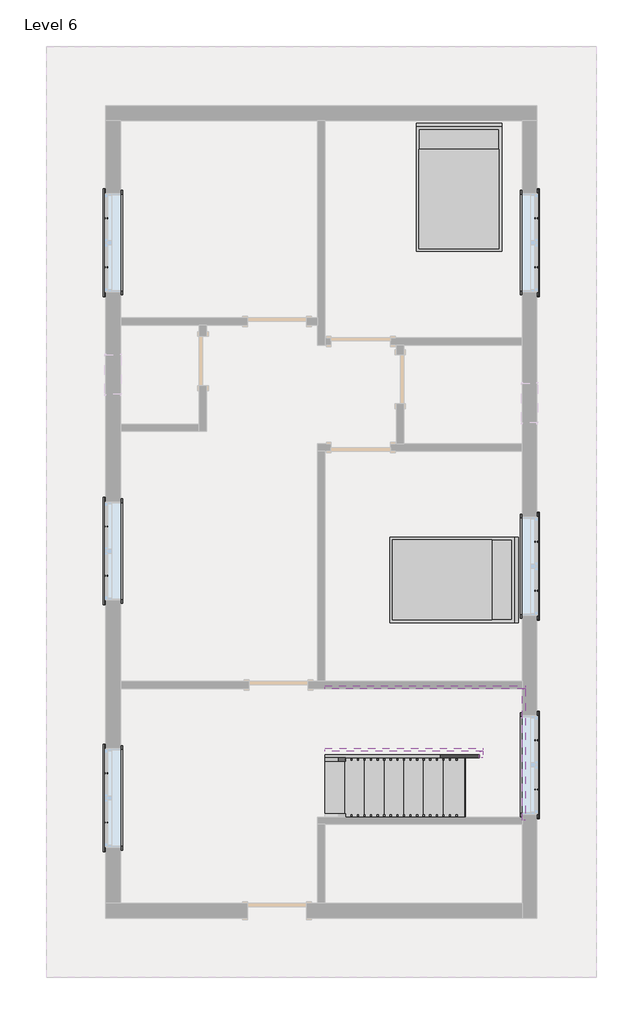
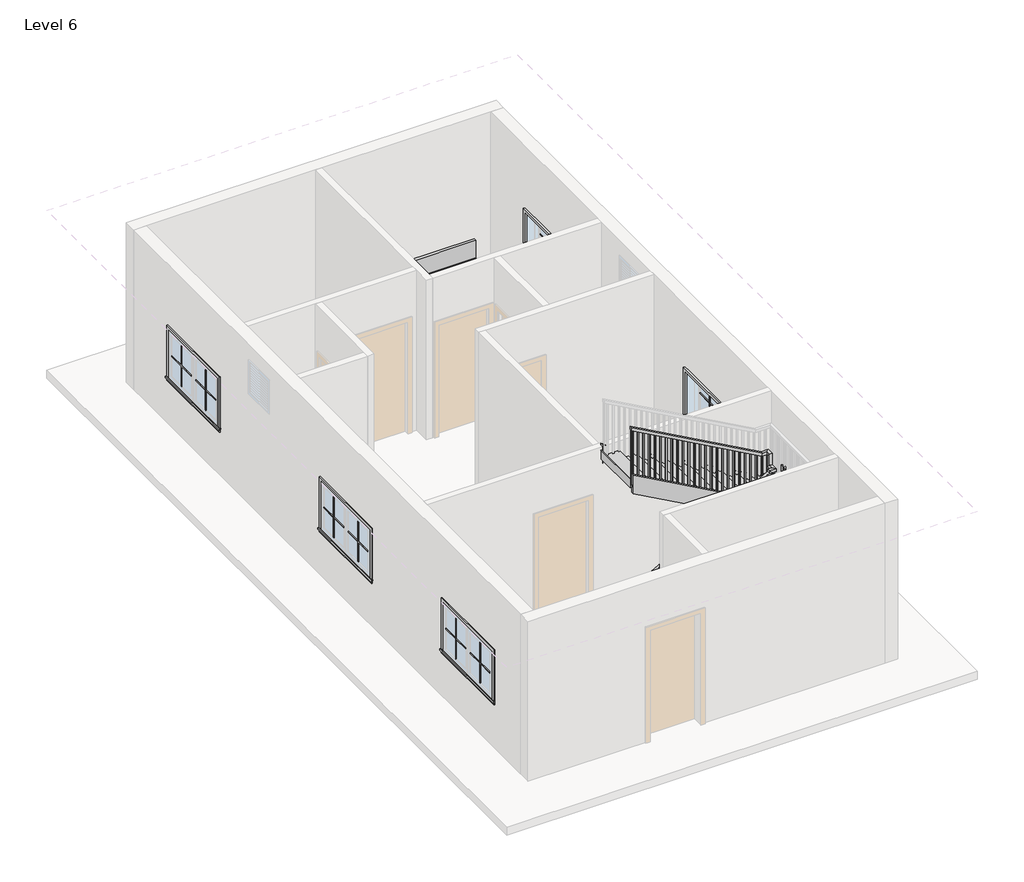
# One storey, part 3 of 3: 24 proxies, 6 members, 2 furniture elements, 1 railing, 1 stair flight.
"""IFC4 building model written with IfcOpenShell, lengths in millimetres."""

from ifc_helpers import new_model, si_unit, frame, origin, place, context, project, spatial, polyline, outline, extrude, faceted_brep, transform, mapped, element, save
from components import muntin_pattern_2x2_muntin_pattern_2x2_9352d081, muntin_pattern_2x2_muntin_pattern_2x2_5c2cbe28, trim_window_exterior_flat_with_sill_979bde60, trim_window_interior_flat_picture_frame_7883d11b, bed_17739_bed_17739_15c61121, stair_flight_3ef849b5

model = new_model("IFC4")

# Units and contexts
model_context = context("Model", 3, world=origin())
ifc_project = project(units=[si_unit("LENGTHUNIT", "METRE", prefix="MILLI")], contexts=[model_context])

# Site, building, storey
site = spatial("IfcSite", under=ifc_project)
building = spatial("IfcBuilding", under=site)
storey = spatial("IfcBuildingStorey", under=building, Name="Level 6", Elevation=15849.6)

# Proxies
placement = place(None, origin())
muntin_pattern_2x2_muntin_pattern_2x2_shape = muntin_pattern_2x2_muntin_pattern_2x2_9352d081(model_context)
element("IfcBuildingElementProxy", 1, Name="Muntin Pattern_2x2 : Muntin Pattern_2x2", ObjectType="Muntin Pattern_2x2 : Muntin Pattern_2x2", at=placement, inside=storey, context=model_context, shape_type="MappedRepresentation", body=[
    mapped(muntin_pattern_2x2_muntin_pattern_2x2_shape, transform((-4579.34688, 3675.02881, 16833.85), x_axis=(0.0, 1.0, 0.0), y_axis=(-1.0, 0.0, 0.0), z_axis=(0.0, 0.0, 1.0))),
])
element("IfcBuildingElementProxy", 2, Name="Muntin Pattern_2x2 : Muntin Pattern_2x2", ObjectType="Muntin Pattern_2x2 : Muntin Pattern_2x2", at=placement, inside=storey, context=model_context, shape_type="MappedRepresentation", body=[
    mapped(muntin_pattern_2x2_muntin_pattern_2x2_shape, transform((-4579.34688, -1087.47119, 16833.85), x_axis=(0.0, 1.0, 0.0), y_axis=(-1.0, 0.0, 0.0), z_axis=(0.0, 0.0, 1.0))),
])
element("IfcBuildingElementProxy", 3, Name="Muntin Pattern_2x2 : Muntin Pattern_2x2", ObjectType="Muntin Pattern_2x2 : Muntin Pattern_2x2", at=placement, inside=storey, context=model_context, shape_type="MappedRepresentation", body=[
    mapped(muntin_pattern_2x2_muntin_pattern_2x2_shape, transform((-4579.34688, -4900.64619, 16833.85), x_axis=(0.0, 1.0, 0.0), y_axis=(-1.0, 0.0, 0.0), z_axis=(0.0, 0.0, 1.0))),
])
element("IfcBuildingElementProxy", 4, Name="Muntin Pattern_2x2 : Muntin Pattern_2x2", ObjectType="Muntin Pattern_2x2 : Muntin Pattern_2x2", at=placement, inside=storey, context=model_context, shape_type="MappedRepresentation", body=[
    mapped(muntin_pattern_2x2_muntin_pattern_2x2_shape, transform((2069.10312, -3630.64619, 16833.85), x_axis=(0.0, -1.0, 0.0), y_axis=(1.0, 0.0, 0.0), z_axis=(0.0, 0.0, 1.0))),
])
element("IfcBuildingElementProxy", 5, Name="Muntin Pattern_2x2 : Muntin Pattern_2x2", ObjectType="Muntin Pattern_2x2 : Muntin Pattern_2x2", at=placement, inside=storey, context=model_context, shape_type="MappedRepresentation", body=[
    mapped(muntin_pattern_2x2_muntin_pattern_2x2_shape, transform((2069.10312, 4433.85381, 16833.85), x_axis=(0.0, -1.0, 0.0), y_axis=(1.0, 0.0, 0.0), z_axis=(0.0, 0.0, 1.0))),
])
element("IfcBuildingElementProxy", 6, Name="Muntin Pattern_2x2 : Muntin Pattern_2x2", ObjectType="Muntin Pattern_2x2 : Muntin Pattern_2x2", at=placement, inside=storey, context=model_context, shape_type="MappedRepresentation", body=[
    mapped(muntin_pattern_2x2_muntin_pattern_2x2_shape, transform((2069.10312, -563.59619, 16833.85), x_axis=(0.0, -1.0, 0.0), y_axis=(1.0, 0.0, 0.0), z_axis=(0.0, 0.0, 1.0))),
])
muntin_pattern_2x2_muntin_pattern_2x2_2_shape = muntin_pattern_2x2_muntin_pattern_2x2_5c2cbe28(model_context)
element("IfcBuildingElementProxy", 7, Name="Muntin Pattern_2x2 : Muntin Pattern_2x2", ObjectType="Muntin Pattern_2x2 : Muntin Pattern_2x2", at=placement, inside=storey, context=model_context, shape_type="MappedRepresentation", body=[
    mapped(muntin_pattern_2x2_muntin_pattern_2x2_2_shape, transform((-4579.34688, 4433.85381, 16833.85), x_axis=(0.0, -1.0, 0.0), y_axis=(1.0, 0.0, 0.0), z_axis=(0.0, 0.0, 1.0))),
])
element("IfcBuildingElementProxy", 8, Name="Muntin Pattern_2x2 : Muntin Pattern_2x2", ObjectType="Muntin Pattern_2x2 : Muntin Pattern_2x2", at=placement, inside=storey, context=model_context, shape_type="MappedRepresentation", body=[
    mapped(muntin_pattern_2x2_muntin_pattern_2x2_2_shape, transform((-4579.34688, -328.64619, 16833.85), x_axis=(0.0, -1.0, 0.0), y_axis=(1.0, 0.0, 0.0), z_axis=(0.0, 0.0, 1.0))),
])
element("IfcBuildingElementProxy", 9, Name="Muntin Pattern_2x2 : Muntin Pattern_2x2", ObjectType="Muntin Pattern_2x2 : Muntin Pattern_2x2", at=placement, inside=storey, context=model_context, shape_type="MappedRepresentation", body=[
    mapped(muntin_pattern_2x2_muntin_pattern_2x2_2_shape, transform((-4579.34688, -4141.82119, 16833.85), x_axis=(0.0, -1.0, 0.0), y_axis=(1.0, 0.0, 0.0), z_axis=(0.0, 0.0, 1.0))),
])
element("IfcBuildingElementProxy", 10, Name="Muntin Pattern_2x2 : Muntin Pattern_2x2", ObjectType="Muntin Pattern_2x2 : Muntin Pattern_2x2", at=placement, inside=storey, context=model_context, shape_type="MappedRepresentation", body=[
    mapped(muntin_pattern_2x2_muntin_pattern_2x2_2_shape, transform((2069.10312, -4389.47119, 16833.85), x_axis=(0.0, 1.0, 0.0), y_axis=(-1.0, 0.0, 0.0), z_axis=(0.0, 0.0, 1.0))),
])
element("IfcBuildingElementProxy", 11, Name="Muntin Pattern_2x2 : Muntin Pattern_2x2", ObjectType="Muntin Pattern_2x2 : Muntin Pattern_2x2", at=placement, inside=storey, context=model_context, shape_type="MappedRepresentation", body=[
    mapped(muntin_pattern_2x2_muntin_pattern_2x2_2_shape, transform((2069.10312, 3675.02881, 16833.85), x_axis=(0.0, 1.0, 0.0), y_axis=(-1.0, 0.0, 0.0), z_axis=(0.0, 0.0, 1.0))),
])
element("IfcBuildingElementProxy", 12, Name="Muntin Pattern_2x2 : Muntin Pattern_2x2", ObjectType="Muntin Pattern_2x2 : Muntin Pattern_2x2", at=placement, inside=storey, context=model_context, shape_type="MappedRepresentation", body=[
    mapped(muntin_pattern_2x2_muntin_pattern_2x2_2_shape, transform((2069.10312, -1322.42119, 16833.85), x_axis=(0.0, 1.0, 0.0), y_axis=(-1.0, 0.0, 0.0), z_axis=(0.0, 0.0, 1.0))),
])
trim_window_exterior_flat_with_sill_shape = trim_window_exterior_flat_with_sill_979bde60(model_context)
element("IfcBuildingElementProxy", 13, Name="Trim-Window-Exterior-Flat : with Sill", ObjectType="Trim-Window-Exterior-Flat : with Sill", at=placement, inside=storey, context=model_context, shape_type="MappedRepresentation", body=[
    mapped(trim_window_exterior_flat_with_sill_shape, transform((-4588.87188, 4054.44131, 17678.4), x_axis=(0.0, -1.0, 0.0), y_axis=(0.0, 0.0, 1.0), z_axis=(-1.0, 0.0, 0.0))),
])
element("IfcBuildingElementProxy", 14, Name="Trim-Window-Exterior-Flat : with Sill", ObjectType="Trim-Window-Exterior-Flat : with Sill", at=placement, inside=storey, context=model_context, shape_type="MappedRepresentation", body=[
    mapped(trim_window_exterior_flat_with_sill_shape, transform((-4588.87188, -708.05869, 17678.4), x_axis=(0.0, -1.0, 0.0), y_axis=(0.0, 0.0, 1.0), z_axis=(-1.0, 0.0, 0.0))),
])
element("IfcBuildingElementProxy", 15, Name="Trim-Window-Exterior-Flat : with Sill", ObjectType="Trim-Window-Exterior-Flat : with Sill", at=placement, inside=storey, context=model_context, shape_type="MappedRepresentation", body=[
    mapped(trim_window_exterior_flat_with_sill_shape, transform((-4588.87188, -4521.23369, 17678.4), x_axis=(0.0, -1.0, 0.0), y_axis=(0.0, 0.0, 1.0), z_axis=(-1.0, 0.0, 0.0))),
])
element("IfcBuildingElementProxy", 16, Name="Trim-Window-Exterior-Flat : with Sill", ObjectType="Trim-Window-Exterior-Flat : with Sill", at=placement, inside=storey, context=model_context, shape_type="MappedRepresentation", body=[
    mapped(trim_window_exterior_flat_with_sill_shape, transform((2078.62812, -4010.05869, 17678.4), x_axis=(0.0, 1.0, 0.0), y_axis=(0.0, 0.0, 1.0), z_axis=(1.0, 0.0, 0.0))),
])
element("IfcBuildingElementProxy", 17, Name="Trim-Window-Exterior-Flat : with Sill", ObjectType="Trim-Window-Exterior-Flat : with Sill", at=placement, inside=storey, context=model_context, shape_type="MappedRepresentation", body=[
    mapped(trim_window_exterior_flat_with_sill_shape, transform((2078.62812, 4054.44131, 17678.4), x_axis=(0.0, 1.0, 0.0), y_axis=(0.0, 0.0, 1.0), z_axis=(1.0, 0.0, 0.0))),
])
element("IfcBuildingElementProxy", 18, Name="Trim-Window-Exterior-Flat : with Sill", ObjectType="Trim-Window-Exterior-Flat : with Sill", at=placement, inside=storey, context=model_context, shape_type="MappedRepresentation", body=[
    mapped(trim_window_exterior_flat_with_sill_shape, transform((2078.62812, -943.00869, 17678.4), x_axis=(0.0, 1.0, 0.0), y_axis=(0.0, 0.0, 1.0), z_axis=(1.0, 0.0, 0.0))),
])
trim_window_interior_flat_picture_frame_shape = trim_window_interior_flat_picture_frame_7883d11b(model_context)
element("IfcBuildingElementProxy", 19, Name="Trim-Window-Interior-Flat : Picture Frame", ObjectType="Trim-Window-Interior-Flat : Picture Frame", at=placement, inside=storey, context=model_context, shape_type="MappedRepresentation", body=[
    mapped(trim_window_interior_flat_picture_frame_shape, transform((-4360.27188, 4054.44131, 17678.4), x_axis=(0.0, 1.0, 0.0), y_axis=(0.0, 0.0, 1.0), z_axis=(1.0, 0.0, 0.0))),
])
element("IfcBuildingElementProxy", 20, Name="Trim-Window-Interior-Flat : Picture Frame", ObjectType="Trim-Window-Interior-Flat : Picture Frame", at=placement, inside=storey, context=model_context, shape_type="MappedRepresentation", body=[
    mapped(trim_window_interior_flat_picture_frame_shape, transform((-4360.27188, -708.05869, 17678.4), x_axis=(0.0, 1.0, 0.0), y_axis=(0.0, 0.0, 1.0), z_axis=(1.0, 0.0, 0.0))),
])
element("IfcBuildingElementProxy", 21, Name="Trim-Window-Interior-Flat : Picture Frame", ObjectType="Trim-Window-Interior-Flat : Picture Frame", at=placement, inside=storey, context=model_context, shape_type="MappedRepresentation", body=[
    mapped(trim_window_interior_flat_picture_frame_shape, transform((-4360.27188, -4521.23369, 17678.4), x_axis=(0.0, 1.0, 0.0), y_axis=(0.0, 0.0, 1.0), z_axis=(1.0, 0.0, 0.0))),
])
element("IfcBuildingElementProxy", 22, Name="Trim-Window-Interior-Flat : Picture Frame", ObjectType="Trim-Window-Interior-Flat : Picture Frame", at=placement, inside=storey, context=model_context, shape_type="MappedRepresentation", body=[
    mapped(trim_window_interior_flat_picture_frame_shape, transform((1850.02812, -4010.05869, 17678.4), x_axis=(0.0, -1.0, 0.0), y_axis=(0.0, 0.0, 1.0), z_axis=(-1.0, 0.0, 0.0))),
])
element("IfcBuildingElementProxy", 23, Name="Trim-Window-Interior-Flat : Picture Frame", ObjectType="Trim-Window-Interior-Flat : Picture Frame", at=placement, inside=storey, context=model_context, shape_type="MappedRepresentation", body=[
    mapped(trim_window_interior_flat_picture_frame_shape, transform((1850.02812, 4054.44131, 17678.4), x_axis=(0.0, -1.0, 0.0), y_axis=(0.0, 0.0, 1.0), z_axis=(-1.0, 0.0, 0.0))),
])
element("IfcBuildingElementProxy", 24, Name="Trim-Window-Interior-Flat : Picture Frame", ObjectType="Trim-Window-Interior-Flat : Picture Frame", at=placement, inside=storey, context=model_context, shape_type="MappedRepresentation", body=[
    mapped(trim_window_interior_flat_picture_frame_shape, transform((1850.02812, -943.00869, 17678.4), x_axis=(0.0, -1.0, 0.0), y_axis=(0.0, 0.0, 1.0), z_axis=(-1.0, 0.0, 0.0))),
])

# Furniture
bed_17739_bed_17739_shape = bed_17739_bed_17739_15c61121(model_context)
element("IfcFurniture", 25, ObjectType="Bed_17739 : Bed_17739", at=placement, inside=storey, context=model_context, shape_type="MappedRepresentation", body=[
    mapped(bed_17739_bed_17739_shape, transform((872.12812, 4886.29131, 15849.6), x_axis=(1.0, 0.0, 0.0), y_axis=(0.0, 1.0, 0.0), z_axis=(0.0, 0.0, 1.0))),
])
element("IfcFurniture", 26, ObjectType="Bed_17739 : Bed_17739", at=placement, inside=storey, context=model_context, shape_type="MappedRepresentation", body=[
    mapped(bed_17739_bed_17739_shape, transform((770.52812, -1152.55869, 15849.6), x_axis=(0.0, -1.0, 0.0), y_axis=(1.0, 0.0, 0.0), z_axis=(0.0, 0.0, 1.0))),
])

# Members
element("IfcMember", 27, ObjectType="Stringer - 2\" Width", at=placement, inside=storey, context=model_context, shape_type="SweptSolid", body=[
    extrude(outline(polyline([(16057.1983948, -1197.97188), (15849.6, -1197.97188), (15849.6, -944.0273772), (17034.9641651, 1189.62812), (17383.6428392, 1189.62812), (16057.1983948, -1197.97188)])), frame((0.0, -3902.10869, 0.0), z_axis=(0.0, 1.0, 0.0), x_axis=(0.0, 0.0, 1.0)), (0.0, 0.0, 1.0), 50.8),
])
element("IfcMember", 28, ObjectType="Stringer - 2\" Width", at=placement, inside=storey, context=model_context, shape_type="SweptSolid", body=[
    extrude(outline(polyline([(1240.42812, -3902.10869), (1189.62812, -3902.10869), (1189.62812, -3800.50869), (1240.42812, -3800.50869), (1240.42812, -3902.10869)])), frame((0.0, 0.0, 17145.0), z_axis=(0.0, 0.0, 1.0), x_axis=(1.0, 0.0, 0.0)), (0.0, 0.0, 1.0), 304.8),
])
element("IfcMember", 29, ObjectType="Stringer - 2\" Width", at=placement, inside=storey, context=model_context, shape_type="SweptSolid", body=[
    extrude(outline(polyline([(17232.5197207, 1240.42812), (17581.1983948, 1240.42812), (18935.8650614, -1197.97188), (18587.1863873, -1197.97188), (17232.5197207, 1240.42812)])), frame((0.0, -3800.50869, 0.0), z_axis=(0.0, 1.0, 0.0), x_axis=(0.0, 0.0, 1.0)), (0.0, 0.0, 1.0), 50.8),
])
element("IfcMember", 30, ObjectType="Stringer - 2\" Width", at=placement, inside=storey, context=model_context, shape_type="SweptSolid", body=[
    extrude(outline(polyline([(16057.1983948, -1197.97188), (15849.6, -1197.97188), (15849.6, -944.0273772), (17401.853054, 1850.02812), (17449.8, 1850.02812), (17449.8, 1308.7110094), (16057.1983948, -1197.97188)])), frame((0.0, -4867.30869, 0.0), z_axis=(0.0, 1.0, 0.0), x_axis=(0.0, 0.0, 1.0)), (0.0, 0.0, 1.0), 50.8),
])
element("IfcMember", 31, ObjectType="Stringer - 2\" Width", at=placement, inside=storey, context=model_context, shape_type="SweptSolid", body=[
    extrude(outline(polyline([(1900.82812, -4867.30869), (1850.02812, -4867.30869), (1850.02812, -2835.30869), (1900.82812, -2835.30869), (1900.82812, -4867.30869)])), frame((0.0, 0.0, 17145.0), z_axis=(0.0, 0.0, 1.0), x_axis=(1.0, 0.0, 0.0)), (0.0, 0.0, 1.0), 304.8),
])
element("IfcMember", 32, ObjectType="Stringer - 2\" Width", at=placement, inside=storey, context=model_context, shape_type="SweptSolid", body=[
    extrude(outline(polyline([(17145.0, 1900.82812), (17214.3095059, 1900.82812), (18935.8650614, -1197.97188), (18587.1863873, -1197.97188), (17145.0, 1397.9636172), (17145.0, 1900.82812)])), frame((0.0, -2835.30869, 0.0), z_axis=(0.0, 1.0, 0.0), x_axis=(0.0, 0.0, 1.0)), (0.0, 0.0, 1.0), 50.8),
])

# Railing
element("IfcRailing", 33, ObjectType="Handrail - Rectangular", at=placement, inside=storey, context=model_context, shape_type="SolidModel", body=[
    faceted_brep([(-1197.97188, -3902.10869, 16933.3333333), (-1197.97188, -3902.10869, 16875.220221), (-1197.97188, -3952.90869, 16875.220221), (-1197.97188, -3952.90869, 16933.3333333), (1164.22812, -3902.10869, 18245.6666667), (1215.02812, -3902.10869, 18215.7757765), (1215.02812, -3952.90869, 18215.7757765), (1164.22812, -3952.90869, 18245.6666667), (1164.22812, -3902.10869, 18288.0), (1215.02812, -3902.10869, 18237.2), (1215.02812, -3952.90869, 18237.2), (1164.22812, -3952.90869, 18288.0), (1240.42812, -3902.10869, 18288.0), (1240.42812, -3902.10869, 18237.2), (1291.22812, -3952.90869, 18237.2), (1291.22812, -3952.90869, 18288.0), (1240.42812, -3825.90869, 18288.0), (1240.42812, -3775.10869, 18237.2), (1291.22812, -3775.10869, 18237.2), (1291.22812, -3825.90869, 18288.0), (1240.42812, -3825.90869, 18499.6666667), (1240.42812, -3775.10869, 18448.8666667), (1291.22812, -3775.10869, 18448.8666667), (1291.22812, -3825.90869, 18499.6666667), (1240.42812, -3749.70869, 18499.6666667), (1240.42812, -3749.70869, 18448.8666667), (1291.22812, -3698.90869, 18448.8666667), (1291.22812, -3698.90869, 18499.6666667), (1164.22812, -3749.70869, 18499.6666667), (1151.0645177, -3749.70869, 18448.8666667), (1151.0645177, -3698.90869, 18448.8666667), (1164.22812, -3698.90869, 18499.6666667), (-1197.97188, -3749.70869, 19812.0), (-1197.97188, -3698.90869, 19812.0), (-1197.97188, -3698.90869, 19753.8868876), (-1197.97188, -3749.70869, 19753.8868876)], [[[0, 1, 2, 3]], [[1, 0, 4, 5]], [[2, 1, 5, 6]], [[3, 2, 6, 7]], [[0, 3, 7, 4]], [[5, 4, 8, 9]], [[6, 5, 9, 10]], [[7, 6, 10, 11]], [[4, 7, 11, 8]], [[9, 8, 12, 13]], [[10, 9, 13, 14]], [[11, 10, 14, 15]], [[8, 11, 15, 12]], [[13, 12, 16, 17]], [[14, 13, 17, 18]], [[15, 14, 18, 19]], [[12, 15, 19, 16]], [[17, 16, 20, 21]], [[18, 17, 21, 22]], [[19, 18, 22, 23]], [[16, 19, 23, 20]], [[21, 20, 24, 25]], [[22, 21, 25, 26]], [[23, 22, 26, 27]], [[20, 23, 27, 24]], [[25, 24, 28, 29]], [[26, 25, 29, 30]], [[27, 26, 30, 31]], [[24, 27, 31, 28]], [[32, 33, 34, 35]], [[29, 28, 32, 35]], [[30, 29, 35, 34]], [[31, 30, 34, 33]], [[28, 31, 33, 32]]]),
    extrude(outline(polyline([(19745.0674432, -1182.09688), (18728.2666667, -1182.09688), (18728.2666667, -1163.04688), (19734.4841099, -1163.04688), (19745.0674432, -1182.09688)])), frame((0.0, -3733.83369, 0.0), z_axis=(0.0, 1.0, 0.0), x_axis=(0.0, 0.0, 1.0)), (0.0, 0.0, 1.0), 19.05),
    extrude(outline(polyline([(19688.6229988, -1080.49688), (18728.2666667, -1080.49688), (18728.2666667, -1061.44688), (19678.0396654, -1061.44688), (19688.6229988, -1080.49688)])), frame((0.0, -3733.83369, 0.0), z_axis=(0.0, 1.0, 0.0), x_axis=(0.0, 0.0, 1.0)), (0.0, 0.0, 1.0), 19.05),
    extrude(outline(polyline([(19632.1785543, -978.89688), (18728.2666667, -978.89688), (18728.2666667, -959.84688), (19621.595221, -959.84688), (19632.1785543, -978.89688)])), frame((0.0, -3733.83369, 0.0), z_axis=(0.0, 1.0, 0.0), x_axis=(0.0, 0.0, 1.0)), (0.0, 0.0, 1.0), 19.05),
    extrude(outline(polyline([(19575.7341099, -877.29688), (18558.9333333, -877.29688), (18558.9333333, -858.24688), (19565.1507765, -858.24688), (19575.7341099, -877.29688)])), frame((0.0, -3733.83369, 0.0), z_axis=(0.0, 1.0, 0.0), x_axis=(0.0, 0.0, 1.0)), (0.0, 0.0, 1.0), 19.05),
    extrude(outline(polyline([(19519.2896654, -775.69688), (18558.9333333, -775.69688), (18558.9333333, -756.64688), (19508.7063321, -756.64688), (19519.2896654, -775.69688)])), frame((0.0, -3733.83369, 0.0), z_axis=(0.0, 1.0, 0.0), x_axis=(0.0, 0.0, 1.0)), (0.0, 0.0, 1.0), 19.05),
    extrude(outline(polyline([(19462.845221, -674.09688), (18558.9333333, -674.09688), (18558.9333333, -655.04688), (19452.2618876, -655.04688), (19462.845221, -674.09688)])), frame((0.0, -3733.83369, 0.0), z_axis=(0.0, 1.0, 0.0), x_axis=(0.0, 0.0, 1.0)), (0.0, 0.0, 1.0), 19.05),
    extrude(outline(polyline([(19406.4007765, -572.49688), (18389.6, -572.49688), (18389.6, -553.44688), (19395.8174432, -553.44688), (19406.4007765, -572.49688)])), frame((0.0, -3733.83369, 0.0), z_axis=(0.0, 1.0, 0.0), x_axis=(0.0, 0.0, 1.0)), (0.0, 0.0, 1.0), 19.05),
    extrude(outline(polyline([(19349.9563321, -470.89688), (18389.6, -470.89688), (18389.6, -451.84688), (19339.3729988, -451.84688), (19349.9563321, -470.89688)])), frame((0.0, -3733.83369, 0.0), z_axis=(0.0, 1.0, 0.0), x_axis=(0.0, 0.0, 1.0)), (0.0, 0.0, 1.0), 19.05),
    extrude(outline(polyline([(19293.5118876, -369.29688), (18389.6, -369.29688), (18389.6, -350.24688), (19282.9285543, -350.24688), (19293.5118876, -369.29688)])), frame((0.0, -3733.83369, 0.0), z_axis=(0.0, 1.0, 0.0), x_axis=(0.0, 0.0, 1.0)), (0.0, 0.0, 1.0), 19.05),
    extrude(outline(polyline([(19237.0674432, -267.69688), (18220.2666667, -267.69688), (18220.2666667, -248.64688), (19226.4841099, -248.64688), (19237.0674432, -267.69688)])), frame((0.0, -3733.83369, 0.0), z_axis=(0.0, 1.0, 0.0), x_axis=(0.0, 0.0, 1.0)), (0.0, 0.0, 1.0), 19.05),
    extrude(outline(polyline([(19180.6229988, -166.09688), (18220.2666667, -166.09688), (18220.2666667, -147.04688), (19170.0396654, -147.04688), (19180.6229988, -166.09688)])), frame((0.0, -3733.83369, 0.0), z_axis=(0.0, 1.0, 0.0), x_axis=(0.0, 0.0, 1.0)), (0.0, 0.0, 1.0), 19.05),
    extrude(outline(polyline([(19124.1785543, -64.49688), (18220.2666667, -64.49688), (18220.2666667, -45.44688), (19113.595221, -45.44688), (19124.1785543, -64.49688)])), frame((0.0, -3733.83369, 0.0), z_axis=(0.0, 1.0, 0.0), x_axis=(0.0, 0.0, 1.0)), (0.0, 0.0, 1.0), 19.05),
    extrude(outline(polyline([(19067.7341099, 37.10312), (18050.9333333, 37.10312), (18050.9333333, 56.15312), (19057.1507765, 56.15312), (19067.7341099, 37.10312)])), frame((0.0, -3733.83369, 0.0), z_axis=(0.0, 1.0, 0.0), x_axis=(0.0, 0.0, 1.0)), (0.0, 0.0, 1.0), 19.05),
    extrude(outline(polyline([(19011.2896654, 138.70312), (18050.9333333, 138.70312), (18050.9333333, 157.75312), (19000.7063321, 157.75312), (19011.2896654, 138.70312)])), frame((0.0, -3733.83369, 0.0), z_axis=(0.0, 1.0, 0.0), x_axis=(0.0, 0.0, 1.0)), (0.0, 0.0, 1.0), 19.05),
    extrude(outline(polyline([(18954.845221, 240.30312), (18050.9333333, 240.30312), (18050.9333333, 259.35312), (18944.2618876, 259.35312), (18954.845221, 240.30312)])), frame((0.0, -3733.83369, 0.0), z_axis=(0.0, 1.0, 0.0), x_axis=(0.0, 0.0, 1.0)), (0.0, 0.0, 1.0), 19.05),
    extrude(outline(polyline([(18898.4007765, 341.90312), (17881.6, 341.90312), (17881.6, 360.95312), (18887.8174432, 360.95312), (18898.4007765, 341.90312)])), frame((0.0, -3733.83369, 0.0), z_axis=(0.0, 1.0, 0.0), x_axis=(0.0, 0.0, 1.0)), (0.0, 0.0, 1.0), 19.05),
    extrude(outline(polyline([(18841.9563321, 443.50312), (17881.6, 443.50312), (17881.6, 462.55312), (18831.3729988, 462.55312), (18841.9563321, 443.50312)])), frame((0.0, -3733.83369, 0.0), z_axis=(0.0, 1.0, 0.0), x_axis=(0.0, 0.0, 1.0)), (0.0, 0.0, 1.0), 19.05),
    extrude(outline(polyline([(18785.5118876, 545.10312), (17881.6, 545.10312), (17881.6, 564.15312), (18774.9285543, 564.15312), (18785.5118876, 545.10312)])), frame((0.0, -3733.83369, 0.0), z_axis=(0.0, 1.0, 0.0), x_axis=(0.0, 0.0, 1.0)), (0.0, 0.0, 1.0), 19.05),
    extrude(outline(polyline([(18729.0674432, 646.70312), (17712.2666667, 646.70312), (17712.2666667, 665.75312), (18718.4841099, 665.75312), (18729.0674432, 646.70312)])), frame((0.0, -3733.83369, 0.0), z_axis=(0.0, 1.0, 0.0), x_axis=(0.0, 0.0, 1.0)), (0.0, 0.0, 1.0), 19.05),
    extrude(outline(polyline([(18672.6229988, 748.30312), (17712.2666667, 748.30312), (17712.2666667, 767.35312), (18662.0396654, 767.35312), (18672.6229988, 748.30312)])), frame((0.0, -3733.83369, 0.0), z_axis=(0.0, 1.0, 0.0), x_axis=(0.0, 0.0, 1.0)), (0.0, 0.0, 1.0), 19.05),
    extrude(outline(polyline([(18616.1785543, 849.90312), (17712.2666667, 849.90312), (17712.2666667, 868.95312), (18605.595221, 868.95312), (18616.1785543, 849.90312)])), frame((0.0, -3733.83369, 0.0), z_axis=(0.0, 1.0, 0.0), x_axis=(0.0, 0.0, 1.0)), (0.0, 0.0, 1.0), 19.05),
    extrude(outline(polyline([(18559.7341099, 951.50312), (17542.9333333, 951.50312), (17542.9333333, 970.55312), (18549.1507765, 970.55312), (18559.7341099, 951.50312)])), frame((0.0, -3733.83369, 0.0), z_axis=(0.0, 1.0, 0.0), x_axis=(0.0, 0.0, 1.0)), (0.0, 0.0, 1.0), 19.05),
    extrude(outline(polyline([(18503.2896654, 1053.10312), (17542.9333333, 1053.10312), (17542.9333333, 1072.15312), (18492.7063321, 1072.15312), (18503.2896654, 1053.10312)])), frame((0.0, -3733.83369, 0.0), z_axis=(0.0, 1.0, 0.0), x_axis=(0.0, 0.0, 1.0)), (0.0, 0.0, 1.0), 19.05),
    extrude(outline(polyline([(18446.845221, 1154.70312), (17542.9333333, 1154.70312), (17542.9333333, 1173.75312), (18436.2618876, 1173.75312), (18446.845221, 1154.70312)])), frame((0.0, -3733.83369, 0.0), z_axis=(0.0, 1.0, 0.0), x_axis=(0.0, 0.0, 1.0)), (0.0, 0.0, 1.0), 19.05),
    extrude(outline(polyline([(1256.30312, -3835.43369), (1256.30312, -3816.38369), (1275.35312, -3816.38369), (1275.35312, -3835.43369), (1256.30312, -3835.43369)])), frame((0.0, 0.0, 17373.6), z_axis=(0.0, 0.0, 1.0), x_axis=(1.0, 0.0, 0.0)), (0.0, 0.0, 1.0), 863.6),
    extrude(outline(polyline([(1230.90312, -3917.98369), (1249.95312, -3917.98369), (1249.95312, -3937.03369), (1230.90312, -3937.03369), (1230.90312, -3917.98369)])), frame((0.0, 0.0, 17373.6), z_axis=(0.0, 0.0, 1.0), x_axis=(1.0, 0.0, 0.0)), (0.0, 0.0, 1.0), 863.6),
    extrude(outline(polyline([(18168.1507765, 1129.30312), (17204.2666667, 1129.30312), (17204.2666667, 1148.35312), (18178.7341099, 1148.35312), (18168.1507765, 1129.30312)])), frame((0.0, -3937.03369, 0.0), z_axis=(0.0, 1.0, 0.0), x_axis=(0.0, 0.0, 1.0)), (0.0, 0.0, 1.0), 19.05),
    extrude(outline(polyline([(18111.7063321, 1027.70312), (17204.2666667, 1027.70312), (17204.2666667, 1046.75312), (18122.2896654, 1046.75312), (18111.7063321, 1027.70312)])), frame((0.0, -3937.03369, 0.0), z_axis=(0.0, 1.0, 0.0), x_axis=(0.0, 0.0, 1.0)), (0.0, 0.0, 1.0), 19.05),
    extrude(outline(polyline([(18055.2618876, 926.10312), (17204.2666667, 926.10312), (17204.2666667, 945.15312), (18065.845221, 945.15312), (18055.2618876, 926.10312)])), frame((0.0, -3937.03369, 0.0), z_axis=(0.0, 1.0, 0.0), x_axis=(0.0, 0.0, 1.0)), (0.0, 0.0, 1.0), 19.05),
    extrude(outline(polyline([(17998.8174432, 824.50312), (17034.9333333, 824.50312), (17034.9333333, 843.55312), (18009.4007765, 843.55312), (17998.8174432, 824.50312)])), frame((0.0, -3937.03369, 0.0), z_axis=(0.0, 1.0, 0.0), x_axis=(0.0, 0.0, 1.0)), (0.0, 0.0, 1.0), 19.05),
    extrude(outline(polyline([(17942.3729988, 722.90312), (17034.9333333, 722.90312), (17034.9333333, 741.95312), (17952.9563321, 741.95312), (17942.3729988, 722.90312)])), frame((0.0, -3937.03369, 0.0), z_axis=(0.0, 1.0, 0.0), x_axis=(0.0, 0.0, 1.0)), (0.0, 0.0, 1.0), 19.05),
    extrude(outline(polyline([(17885.9285543, 621.30312), (17034.9333333, 621.30312), (17034.9333333, 640.35312), (17896.5118876, 640.35312), (17885.9285543, 621.30312)])), frame((0.0, -3937.03369, 0.0), z_axis=(0.0, 1.0, 0.0), x_axis=(0.0, 0.0, 1.0)), (0.0, 0.0, 1.0), 19.05),
    extrude(outline(polyline([(17829.4841099, 519.70312), (16865.6, 519.70312), (16865.6, 538.75312), (17840.0674432, 538.75312), (17829.4841099, 519.70312)])), frame((0.0, -3937.03369, 0.0), z_axis=(0.0, 1.0, 0.0), x_axis=(0.0, 0.0, 1.0)), (0.0, 0.0, 1.0), 19.05),
    extrude(outline(polyline([(17773.0396654, 418.10312), (16865.6, 418.10312), (16865.6, 437.15312), (17783.6229988, 437.15312), (17773.0396654, 418.10312)])), frame((0.0, -3937.03369, 0.0), z_axis=(0.0, 1.0, 0.0), x_axis=(0.0, 0.0, 1.0)), (0.0, 0.0, 1.0), 19.05),
    extrude(outline(polyline([(17716.595221, 316.50312), (16865.6, 316.50312), (16865.6, 335.55312), (17727.1785543, 335.55312), (17716.595221, 316.50312)])), frame((0.0, -3937.03369, 0.0), z_axis=(0.0, 1.0, 0.0), x_axis=(0.0, 0.0, 1.0)), (0.0, 0.0, 1.0), 19.05),
    extrude(outline(polyline([(17660.1507765, 214.90312), (16696.2666667, 214.90312), (16696.2666667, 233.95312), (17670.7341099, 233.95312), (17660.1507765, 214.90312)])), frame((0.0, -3937.03369, 0.0), z_axis=(0.0, 1.0, 0.0), x_axis=(0.0, 0.0, 1.0)), (0.0, 0.0, 1.0), 19.05),
    extrude(outline(polyline([(17603.7063321, 113.30312), (16696.2666667, 113.30312), (16696.2666667, 132.35312), (17614.2896654, 132.35312), (17603.7063321, 113.30312)])), frame((0.0, -3937.03369, 0.0), z_axis=(0.0, 1.0, 0.0), x_axis=(0.0, 0.0, 1.0)), (0.0, 0.0, 1.0), 19.05),
    extrude(outline(polyline([(17547.2618876, 11.70312), (16696.2666667, 11.70312), (16696.2666667, 30.75312), (17557.845221, 30.75312), (17547.2618876, 11.70312)])), frame((0.0, -3937.03369, 0.0), z_axis=(0.0, 1.0, 0.0), x_axis=(0.0, 0.0, 1.0)), (0.0, 0.0, 1.0), 19.05),
    extrude(outline(polyline([(17490.8174432, -89.89688), (16526.9333333, -89.89688), (16526.9333333, -70.84688), (17501.4007765, -70.84688), (17490.8174432, -89.89688)])), frame((0.0, -3937.03369, 0.0), z_axis=(0.0, 1.0, 0.0), x_axis=(0.0, 0.0, 1.0)), (0.0, 0.0, 1.0), 19.05),
    extrude(outline(polyline([(17434.3729988, -191.49688), (16526.9333333, -191.49688), (16526.9333333, -172.44688), (17444.9563321, -172.44688), (17434.3729988, -191.49688)])), frame((0.0, -3937.03369, 0.0), z_axis=(0.0, 1.0, 0.0), x_axis=(0.0, 0.0, 1.0)), (0.0, 0.0, 1.0), 19.05),
    extrude(outline(polyline([(17377.9285543, -293.09688), (16526.9333333, -293.09688), (16526.9333333, -274.04688), (17388.5118876, -274.04688), (17377.9285543, -293.09688)])), frame((0.0, -3937.03369, 0.0), z_axis=(0.0, 1.0, 0.0), x_axis=(0.0, 0.0, 1.0)), (0.0, 0.0, 1.0), 19.05),
    extrude(outline(polyline([(17321.4841099, -394.69688), (16357.6, -394.69688), (16357.6, -375.64688), (17332.0674432, -375.64688), (17321.4841099, -394.69688)])), frame((0.0, -3937.03369, 0.0), z_axis=(0.0, 1.0, 0.0), x_axis=(0.0, 0.0, 1.0)), (0.0, 0.0, 1.0), 19.05),
    extrude(outline(polyline([(17265.0396654, -496.29688), (16357.6, -496.29688), (16357.6, -477.24688), (17275.6229988, -477.24688), (17265.0396654, -496.29688)])), frame((0.0, -3937.03369, 0.0), z_axis=(0.0, 1.0, 0.0), x_axis=(0.0, 0.0, 1.0)), (0.0, 0.0, 1.0), 19.05),
    extrude(outline(polyline([(17208.595221, -597.89688), (16357.6, -597.89688), (16357.6, -578.84688), (17219.1785543, -578.84688), (17208.595221, -597.89688)])), frame((0.0, -3937.03369, 0.0), z_axis=(0.0, 1.0, 0.0), x_axis=(0.0, 0.0, 1.0)), (0.0, 0.0, 1.0), 19.05),
    extrude(outline(polyline([(17152.1507765, -699.49688), (16188.2666667, -699.49688), (16188.2666667, -680.44688), (17162.7341099, -680.44688), (17152.1507765, -699.49688)])), frame((0.0, -3937.03369, 0.0), z_axis=(0.0, 1.0, 0.0), x_axis=(0.0, 0.0, 1.0)), (0.0, 0.0, 1.0), 19.05),
    extrude(outline(polyline([(17095.7063321, -801.09688), (16188.2666667, -801.09688), (16188.2666667, -782.04688), (17106.2896654, -782.04688), (17095.7063321, -801.09688)])), frame((0.0, -3937.03369, 0.0), z_axis=(0.0, 1.0, 0.0), x_axis=(0.0, 0.0, 1.0)), (0.0, 0.0, 1.0), 19.05),
    extrude(outline(polyline([(17039.2618876, -902.69688), (16188.2666667, -902.69688), (16188.2666667, -883.64688), (17049.845221, -883.64688), (17039.2618876, -902.69688)])), frame((0.0, -3937.03369, 0.0), z_axis=(0.0, 1.0, 0.0), x_axis=(0.0, 0.0, 1.0)), (0.0, 0.0, 1.0), 19.05),
    extrude(outline(polyline([(16982.8174432, -1004.29688), (16018.9333333, -1004.29688), (16018.9333333, -985.24688), (16993.4007765, -985.24688), (16982.8174432, -1004.29688)])), frame((0.0, -3937.03369, 0.0), z_axis=(0.0, 1.0, 0.0), x_axis=(0.0, 0.0, 1.0)), (0.0, 0.0, 1.0), 19.05),
    extrude(outline(polyline([(16926.3729988, -1105.89688), (16018.9333333, -1105.89688), (16018.9333333, -1086.84688), (16936.9563321, -1086.84688), (16926.3729988, -1105.89688)])), frame((0.0, -3937.03369, 0.0), z_axis=(0.0, 1.0, 0.0), x_axis=(0.0, 0.0, 1.0)), (0.0, 0.0, 1.0), 19.05),
    extrude(outline(polyline([(1256.30312, -3733.83369), (1256.30312, -3714.78369), (1275.35312, -3714.78369), (1275.35312, -3733.83369), (1256.30312, -3733.83369)])), frame((0.0, 0.0, 17373.6), z_axis=(0.0, 0.0, 1.0), x_axis=(1.0, 0.0, 0.0)), (0.0, 0.0, 1.0), 1075.2666667),
    extrude(outline(polyline([(1256.30312, -3917.98369), (1275.35312, -3917.98369), (1275.35312, -3937.03369), (1256.30312, -3937.03369), (1256.30312, -3917.98369)])), frame((0.0, 0.0, 17373.6), z_axis=(0.0, 0.0, 1.0), x_axis=(1.0, 0.0, 0.0)), (0.0, 0.0, 1.0), 863.6),
    extrude(outline(polyline([(19753.8868876, -1197.97188), (18728.2666667, -1197.97188), (18728.2666667, -1178.92188), (19743.3035543, -1178.92188), (19753.8868876, -1197.97188)])), frame((0.0, -3733.83369, 0.0), z_axis=(0.0, 1.0, 0.0), x_axis=(0.0, 0.0, 1.0)), (0.0, 0.0, 1.0), 19.05),
    extrude(outline(polyline([(16875.220221, -1197.97188), (16018.9333333, -1197.97188), (16018.9333333, -1178.92188), (16885.8035543, -1178.92188), (16875.220221, -1197.97188)])), frame((0.0, -3937.03369, 0.0), z_axis=(0.0, 1.0, 0.0), x_axis=(0.0, 0.0, 1.0)), (0.0, 0.0, 1.0), 19.05),
])

# Stair flight
stair_flight_shape = stair_flight_3ef849b5(model_context)
element("IfcStairFlight", 34, ObjectType="2\" Tread 1\" Nosing 1/4\" Riser", at=placement, inside=storey, context=model_context, shape_type="MappedRepresentation", body=[
    mapped(stair_flight_shape, transform((0.0, 0.0, 0.0), x_axis=(1.0, 0.0, 0.0), y_axis=(0.0, 1.0, 0.0), z_axis=(0.0, 0.0, 1.0))),
])

save(model, "model.ifc")

# Revit data of these elements
# Type "Muntin Pattern_2x2 : Muntin Pattern_2x2"
#   Width [instance default] = 4' - 0"
#   Thickness = 0' - 0 1/2"
#   Height [instance default] = 4' - 0"
#   Distance = 0' - 0 3/4"
#   Interior Material [instance default] = none
#   Exterior Material [instance default] = none
#   Default Elevation = 0
# Type "Trim-Window-Exterior-Flat : with Sill"
#   Trim Width = 0' - 2 1/4"
#   Trim Thickness_Picture Frame = 0' - 1 1/4"
#   Trim Thickness_with Sill = 0' - 0 3/4"
#   Sill Thickness = 0' - 1 1/4"
#   Opening Width [instance default] = 2' - 0"
#   Opening Height [instance default] = 3' - 0"
#   Default Elevation = 4' - 0"
#   Sill = yes
#   Picture Frame = no
#   Trim Material [instance default] = none
# Type "Trim-Window-Interior-Flat : Picture Frame"
#   Trim Thickness_Picture Frame = 0' - 1 1/4"
#   Trim Width = 0' - 2 1/4"
#   Trim Thickness_with Sill = 0' - 0 3/4"
#   Sill Thickness = 0' - 1 1/4"
#   Opening Width [instance default] = 2' - 0"
#   Opening Height [instance default] = 3' - 0"
#   Default Elevation = 4' - 0"
#   Sill = no
#   Picture Frame = yes
#   Trim Material [instance default] = none
# Type "Bed_17739 : Bed_17739"
#   Default Elevation = 0
# Type "Handrail - Rectangular"
#   Assembly Code = "C2010400"
#   built-in parameter 1008612 = 0.0416667 (stored number, unit not read)
#   built-in parameter 1008611 = 0.0416667 (stored number, unit not read)
#   built-in parameter 1008609 = 0.333333 (stored number, unit not read)
#   built-in parameter 1008604 = 0.166667 (stored number, unit not read)
#   built-in parameter 1008603 = 0.166667 (stored number, unit not read)
#   Railing Height = 3' - 0"
#   built-in parameter 1008630 = 2
#   built-in parameter 1008610 = 2
#   built-in parameter 1008618 = Baluster - Square : 3/4"
# Elements 1, 2, 3, 4, 5, 6, 7, 8, 9, 10, 11, 12 (IfcBuildingElementProxy, "Muntin Pattern_2x2 : Muntin Pattern_2x2")
#   Width = 2' - 0 5/8"
#   Height = 2' - 6 1/2"
#   Interior Material = Wood - Stained
#   Exterior Material = Clad - White
#   Phase Created = New Construction
#   Materials on its faces: "Clad - White", "Wood - Stained"
# Elements 13, 14, 15, 16, 17, 18 (IfcBuildingElementProxy, "Trim-Window-Exterior-Flat : with Sill")
#   Opening Width = 5' - 0"
#   Opening Height = 3' - 0"
#   Trim Material = Clad - White
#   Phase Created = New Construction
#   Materials on its faces: "Clad - White"
# Elements 19, 20, 21, 22, 23, 24 (IfcBuildingElementProxy, "Trim-Window-Interior-Flat : Picture Frame")
#   Opening Width = 5' - 0"
#   Opening Height = 3' - 0"
#   Trim Material = Wood - Stained
#   Phase Created = New Construction
#   Materials on its faces: "Wood - Stained"
# Elements 25, 26 (IfcFurniture, "Bed_17739 : Bed_17739")
#   Phase Created = New Construction
#   Materials on its faces: "legs", "sheets", "bed frame", "Blanket"
# Elements 27, 28, 29, 30, 31, 32 (IfcMember, "Stringer - 2\" Width")
#   Phase Created = New Construction
# Element 33 (IfcRailing, "Handrail - Rectangular")
#   Phase Created = New Construction
# Element 34 (IfcStairFlight, "2\" Tread 1\" Nosing 1/4\" Riser")
#   Phase Created = New Construction
# Materials
#   "Clad - White": class "Wood", colour RGB 242 242 238, transparency 0, Cost = 0
#   "Wood - Stained": class "Wood", colour RGB 224 178 126, transparency 0, Cost = 0
#   "legs": colour RGB 90 73 37, transparency 0, Cost = 0
#   "sheets": colour RGB 200 195 176, transparency 0, Cost = 0
#   "bed frame": colour RGB 90 73 37, transparency 0, Cost = 0
#   "Blanket": class "System", colour RGB 59 0 1, transparency 0, Cost = 0
